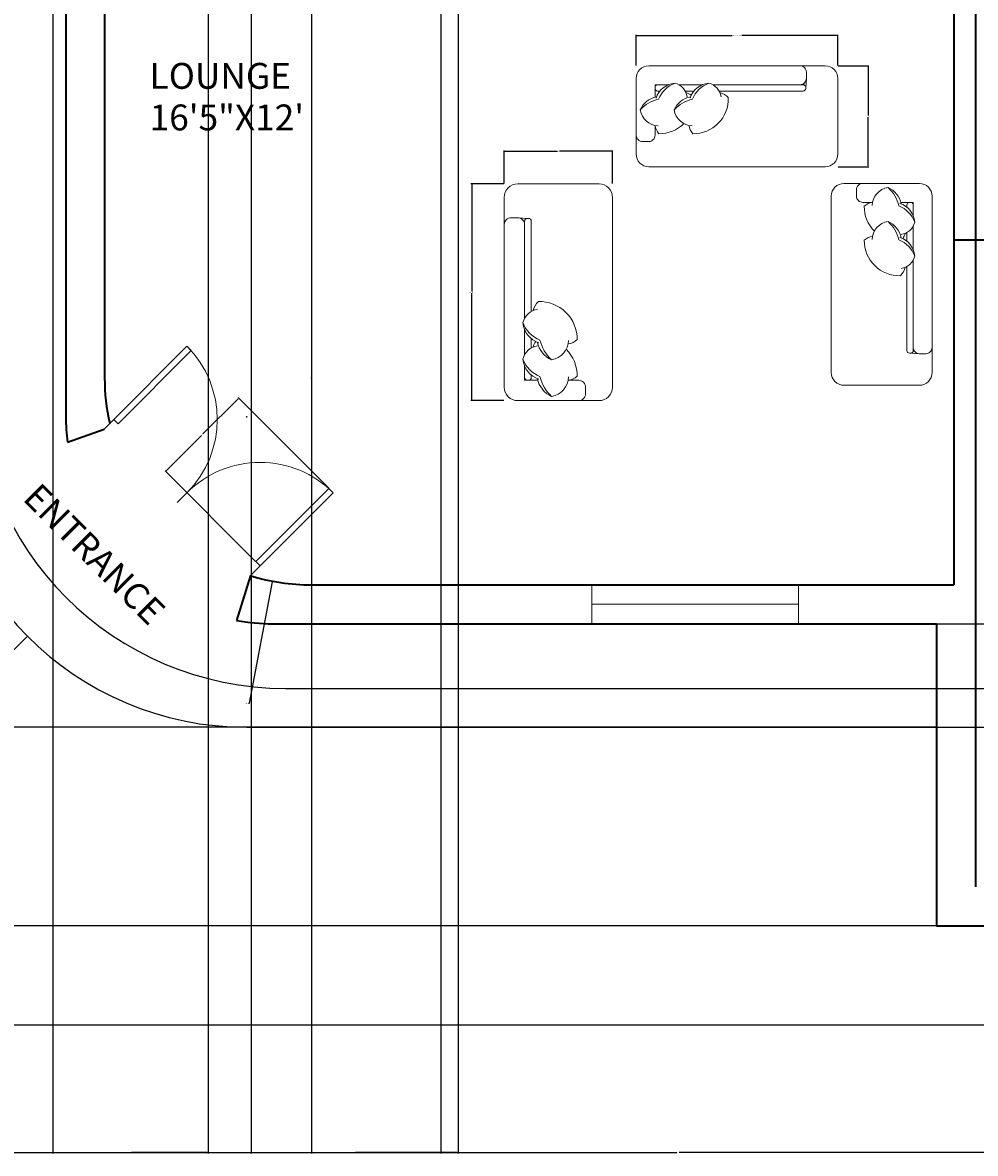
# Model space of a CAD drawing. Units: inches. Extents: x 450 to 1026, y 542 to 1190.
# Tile 4 of 11: x 586 to 807, y 542 to 804. Entities that reach past the tile are written whole.
import ezdxf

# ---------------------------------------------------------------- set-up
doc = ezdxf.new("R2010")
doc.units = ezdxf.units.IN
doc.header["$MEASUREMENT"] = 0
for name, color, linetype, lineweight in [('A-ANNO-DIMS', 2, 'Continuous', 18), ('A-AREA-IDEN', 7, 'Continuous', 18), ('A-DOOR', 4, 'Continuous', 18), ('A-FLOR', 8, 'Continuous', 25), ('A-FURN', 8, 'Continuous', 18), ('A-GLAZ', 4, 'Continuous', 18), ('A-WALL', 7, 'Continuous', 35), ('C-PROP', 7, 'Continuous', 25)]:
    doc.layers.add(name, color=color, linetype=linetype, lineweight=lineweight)
doc.styles.get("Standard").update_dxf_attribs({"font": 'arial.ttf'})
doc.dimstyles.get("Standard").update_dxf_attribs({"dimtxt": 0.18, "dimasz": 0.18, "dimexe": 0.18, "dimexo": 0.0625, "dimgap": 0.09, "dimtad": 0, "dimtih": 1, "dimtoh": 1, "dimdec": 4, "dimzin": 0, "dimdsep": 46, "dimtxsty": 'Standard', "dimcen": 0.09, "dimadec": 0, "dimazin": 0, "dimtfac": 1, "dimtdec": 4, "dimtofl": 0, "dimtmove": 0, "dimatfit": 3, "dimfxl": 1, "dimtolj": 1, "dimtzin": 0, "dimarcsym": 0})

# ---------------------------------------------------------------- blocks, each defined once
blk = doc.blocks.new('*U5')
for p, q in [((0, 0), (0, -100)), ((750, 0), (750, -100))]:
    blk.add_line(p, q)
blk.add_lwpolyline([(0, 0), (0, 750), (43.75, 750), (43.75, 0)], close=True)
blk.add_arc((0, 0), 750, 0, 90)
blk = doc.blocks.new('*U3')
for p, q in [((0, 100), (0, 0)), ((900, 100), (900, 0)), ((0, 50), (900, 50))]:
    blk.add_line(p, q)
blk = doc.blocks.new('DAY BED1')
at = {"color": 0}
blk.add_line((0.3, 0.25), (0.225, 0.2549), dxfattribs=at)
blk.add_lwpolyline([(-0.3, 0, -0.414214), (-0.4, 0.1), (-0.4, 0.1, 0.317837), (-0.4, 0.1, -0.414214), (-0.4, 0.1), (-0.4, 0.1, 1.186185), (-0.4, 0.1, -0.414214), (-0.4, 0.1), (-0.4, 1.5, -0.414214), (-0.3, 1.6), (0.3, 1.6, -0.414214), (0.4, 1.5), (0.4, 0.1, -0.414214), (0.3, 0)], format="xyb", close=True, dxfattribs=at)
for points in [[(-0.0725, 1.45), (-0.15, 1.45, -0.414214), (-0.2, 1.5), (-0.2, 1.55, -0.414214), (-0.15, 1.6)], [(-0.0756, 1.4249, -0.356772), (0.0505, 1.5682, -0.249542), (0.1543, 1.4384, 9.61688)], [(0.0505, 1.5682, -0.14773), (0.1364, 1.422, -0.213343), (0.2624, 1.2931, -0.178662)], [(-0.0725, 1.4501, 0.165541), (-0.1386, 1.4192, 0.200231), (-0.0581, 1.2207, 0.121523)], [(0.1433, 1.4422, -0.306663), (0.2624, 1.2931, -0.30633), (0.1536, 1.1957, 0.872847)], [(0.25, 1.3448), (0.25, 1.45), (0.1517, 1.45, -0.414214)], [(0.2, 1.4118), (0.2, 1.43, -0.414214), (0.22, 1.45), (0.23, 1.45, -0.414214), (0.25, 1.43)], [(0.25, 1.43), (0.25, 1.3448, -0.414214)], [(-0.0756, 1.1556, -0.356772), (0.0505, 1.2988, -0.249542), (0.1543, 1.169, 9.61688)], [(0.0505, 1.2988, -0.14773), (0.1364, 1.1527, -0.213343), (0.2624, 1.0238, -0.178662)], [(0.25, 1.2616), (0.25, 1.0755, -0.414214)], [(-0.0725, 1.1808, 0.165541), (-0.1386, 1.1498, 0.425989), (0.1479, 0.869, 0.121523), (0.1873, 0.9357, -7.115464)], [(0.1433, 1.1729, -0.306663), (0.2624, 1.0238, -0.30633), (0.1536, 0.9263, 0.872847)], [(0.1678, 1.1631, 0.071865), (0.1873, 1.205, -7.115464)], [(0.2, 1.1425), (0.2, 1.2113, -0.414214)], [(0.25, 0.9923), (0.25, 0.2749, -0.414214), (0.23, 0.2549), (0.22, 0.2549, -0.414214), (0.2, 0.2749), (0.2, 0.9419, -0.414214)], [(0.25, 0.3775), (0.25, 0.3, 0.414214), (0.3, 0.25), (0.35, 0.25, 0.414214), (0.4, 0.3)]]:
    blk.add_lwpolyline(points, format="xyb", dxfattribs=at)
for points in [[(0.25, 1.0755), (0.25, 1.2616)], [(0.25, 0.3775), (0.25, 0.9923)]]:
    blk.add_lwpolyline(points, dxfattribs=at)
blk = doc.blocks.new('*D25')
at = {"layer": 'A-ANNO-DIMS', "color": 0, "lineweight": -2, "transparency": 16777216}
for p, q in [((697.29, 766.92), (689.63, 766.92)), ((689.81, 766.74), (689.81, 741.97)), ((689.81, 716.84), (689.81, 741.61)), ((697.29, 716.66), (689.63, 716.66))]:
    blk.add_line(p, q, dxfattribs=at)
at = {"layer": 'A-ANNO-DIMS', "color": 0, "transparency": 16777216}
for points in [[(689.78, 766.74), (689.84, 766.74), (689.81, 766.92)], [(689.78, 716.84), (689.84, 716.84), (689.81, 716.66)]]:
    blk.add_solid(points, dxfattribs=at)
at = {"layer": 'Defpoints', "color": 0, "transparency": 16777216}
for p in [(697.35, 766.92), (689.81, 716.66), (697.35, 716.66)]:
    blk.add_point(p, dxfattribs=at)
at = {"layer": 'A-ANNO-DIMS', "color": 0, "transparency": 16777216, "insert": (689.81, 741.79), "char_height": 0.18, "attachment_point": 5}
blk.add_mtext('\\A1;DAY BED 50', dxfattribs=at)
blk = doc.blocks.new('*D26')
at = {"layer": 'A-ANNO-DIMS', "color": 0, "lineweight": -2, "transparency": 16777216}
for p, q in [((697.35, 766.98), (697.35, 774.64)), ((697.53, 774.46), (709.7, 774.46)), ((722.31, 774.46), (710.14, 774.46)), ((722.49, 766.98), (722.49, 774.64))]:
    blk.add_line(p, q, dxfattribs=at)
at = {"layer": 'A-ANNO-DIMS', "color": 0, "transparency": 16777216}
for points in [[(697.53, 774.49), (697.53, 774.43), (697.35, 774.46)], [(722.31, 774.49), (722.31, 774.43), (722.49, 774.46)]]:
    blk.add_solid(points, dxfattribs=at)
at = {"layer": 'Defpoints', "color": 0, "transparency": 16777216}
for p in [(697.35, 774.46), (697.35, 766.92), (722.49, 766.92)]:
    blk.add_point(p, dxfattribs=at)
at = {"layer": 'A-ANNO-DIMS', "color": 0, "transparency": 16777216, "insert": (709.92, 774.46), "char_height": 0.18, "attachment_point": 5}
blk.add_mtext('\\A1;25', dxfattribs=at)
blk = doc.blocks.new('*D27')
at = {"layer": 'A-ANNO-DIMS', "color": 0, "lineweight": -2, "transparency": 16777216}
for p, q in [((727.96, 794.34), (727.96, 801.47)), ((728.14, 801.29), (750.24, 801.29)), ((774.56, 801.29), (752.46, 801.29)), ((774.74, 794.34), (774.74, 801.47))]:
    blk.add_line(p, q, dxfattribs=at)
at = {"layer": 'A-ANNO-DIMS', "color": 0, "transparency": 16777216}
for points in [[(728.14, 801.32), (728.14, 801.26), (727.96, 801.29)], [(774.56, 801.32), (774.56, 801.26), (774.74, 801.29)]]:
    blk.add_solid(points, dxfattribs=at)
at = {"layer": 'Defpoints', "color": 0, "transparency": 16777216}
for p in [(727.96, 801.29), (727.96, 794.28), (774.74, 794.28)]:
    blk.add_point(p, dxfattribs=at)
at = {"layer": 'A-ANNO-DIMS', "color": 0, "transparency": 16777216, "insert": (751.35, 801.29), "char_height": 0.18, "attachment_point": 5}
blk.add_mtext('\\A1;DAY BED 47 TYP.', dxfattribs=at)
blk = doc.blocks.new('*D28')
at = {"layer": 'A-ANNO-DIMS', "color": 0, "lineweight": -2, "transparency": 16777216}
for p, q in [((774.81, 794.28), (781.94, 794.28)), ((781.76, 794.1), (781.76, 782.76)), ((781.76, 771.07), (781.76, 782.4)), ((774.81, 770.89), (781.94, 770.89))]:
    blk.add_line(p, q, dxfattribs=at)
at = {"layer": 'A-ANNO-DIMS', "color": 0, "transparency": 16777216}
for points in [[(781.73, 794.1), (781.79, 794.1), (781.76, 794.28)], [(781.73, 771.07), (781.79, 771.07), (781.76, 770.89)]]:
    blk.add_solid(points, dxfattribs=at)
at = {"layer": 'Defpoints', "color": 0, "transparency": 16777216}
for p in [(774.74, 794.28), (781.76, 794.28), (774.74, 770.89)]:
    blk.add_point(p, dxfattribs=at)
at = {"layer": 'A-ANNO-DIMS', "color": 0, "transparency": 16777216, "insert": (781.76, 782.58), "char_height": 0.18, "attachment_point": 5}
blk.add_mtext('\\A1;23 TYP.', dxfattribs=at)
blk = doc.blocks.new('*D45')
at = {"layer": 'A-ANNO-DIMS', "color": 0, "lineweight": -2, "transparency": 16777216}
for p, q in [((479.65, 571.88), (479.65, 542.16)), ((995.65, 571.88), (995.65, 542.16)), ((479.83, 542.34), (737.36, 542.34)), ((995.47, 542.34), (737.94, 542.34))]:
    blk.add_line(p, q, dxfattribs=at)
at = {"layer": 'A-ANNO-DIMS', "color": 0, "transparency": 16777216}
for points in [[(479.83, 542.37), (479.83, 542.31), (479.65, 542.34)], [(995.47, 542.37), (995.47, 542.31), (995.65, 542.34)]]:
    blk.add_solid(points, dxfattribs=at)
at = {"layer": 'Defpoints', "color": 0, "transparency": 16777216}
for p in [(479.65, 571.94), (995.65, 571.94), (995.65, 542.34)]:
    blk.add_point(p, dxfattribs=at)
at = {"layer": 'A-ANNO-DIMS', "color": 0, "transparency": 16777216, "insert": (737.65, 542.34), "char_height": 0.18, "attachment_point": 5}
blk.add_mtext('\\A1;516', dxfattribs=at)
blk = doc.blocks.new('*D53')
at = {"layer": 'A-ANNO-DIMS', "color": 0, "lineweight": -2, "transparency": 16777216}
for p, q in [((479.59, 817.94), (449.87, 817.94)), ((450.05, 817.76), (450.05, 706.62)), ((450.05, 595.12), (450.05, 706.26)), ((797.59, 594.94), (449.87, 594.94))]:
    blk.add_line(p, q, dxfattribs=at)
at = {"layer": 'A-ANNO-DIMS', "color": 0, "transparency": 16777216}
for points in [[(450.02, 817.76), (450.08, 817.76), (450.05, 817.94)], [(450.02, 595.12), (450.08, 595.12), (450.05, 594.94)]]:
    blk.add_solid(points, dxfattribs=at)
at = {"layer": 'Defpoints', "color": 0, "transparency": 16777216}
for p in [(479.65, 817.94), (450.05, 594.94), (797.65, 594.94)]:
    blk.add_point(p, dxfattribs=at)
at = {"layer": 'A-ANNO-DIMS', "color": 0, "transparency": 16777216, "insert": (450.05, 706.44), "char_height": 0.18, "attachment_point": 5}
blk.add_mtext('\\A1;223', dxfattribs=at)
blk = doc.blocks.new('*D54')
at = {"layer": 'A-ANNO-DIMS', "color": 0, "lineweight": -2, "transparency": 16777216}
for p, q in [((797.59, 594.94), (449.87, 594.94)), ((450.05, 594.76), (450.05, 583.62)), ((450.05, 572.12), (450.05, 583.26)), ((479.59, 571.94), (449.87, 571.94))]:
    blk.add_line(p, q, dxfattribs=at)
at = {"layer": 'A-ANNO-DIMS', "color": 0, "transparency": 16777216}
for points in [[(450.02, 594.76), (450.08, 594.76), (450.05, 594.94)], [(450.02, 572.12), (450.08, 572.12), (450.05, 571.94)]]:
    blk.add_solid(points, dxfattribs=at)
at = {"layer": 'Defpoints', "color": 0, "transparency": 16777216}
for p in [(797.65, 594.94), (450.05, 571.94), (479.65, 571.94)]:
    blk.add_point(p, dxfattribs=at)
at = {"layer": 'A-ANNO-DIMS', "color": 0, "transparency": 16777216, "insert": (450.05, 583.44), "char_height": 0.18, "attachment_point": 5}
blk.add_mtext('\\A1;23', dxfattribs=at)
blk = doc.blocks.new('*D57')
at = {"layer": 'A-ANNO-DIMS', "color": 0, "lineweight": -2, "transparency": 16777216}
for p, q in [((638.65, 970.88), (638.65, 542.16)), ((686.65, 970.88), (686.65, 542.16)), ((638.83, 542.34), (662.43, 542.34)), ((686.47, 542.34), (662.87, 542.34))]:
    blk.add_line(p, q, dxfattribs=at)
at = {"layer": 'A-ANNO-DIMS', "color": 0, "transparency": 16777216}
for points in [[(638.83, 542.37), (638.83, 542.31), (638.65, 542.34)], [(686.47, 542.37), (686.47, 542.31), (686.65, 542.34)]]:
    blk.add_solid(points, dxfattribs=at)
at = {"layer": 'Defpoints', "color": 0, "transparency": 16777216}
for p in [(638.65, 970.94), (686.65, 970.94), (686.65, 542.34)]:
    blk.add_point(p, dxfattribs=at)
at = {"layer": 'A-ANNO-DIMS', "color": 0, "transparency": 16777216, "insert": (662.65, 542.34), "char_height": 0.18, "attachment_point": 5}
blk.add_mtext('\\A1;48', dxfattribs=at)
blk = doc.blocks.new('*D64')
at = {"layer": 'A-ANNO-DIMS', "color": 0, "lineweight": -2, "transparency": 16777216}
for p, q in [((635.65, 717.11), (627.47, 708.94)), ((656.66, 696.36), (635.65, 717.37)), ((618.93, 700.4), (627.11, 708.58)), ((639.69, 679.38), (618.68, 700.4))]:
    blk.add_line(p, q, dxfattribs=at)
at = {"layer": 'A-ANNO-DIMS', "color": 0, "transparency": 16777216}
for points in [[(635.63, 717.14), (635.67, 717.09), (635.77, 717.24)], [(618.91, 700.42), (618.95, 700.38), (618.8, 700.27)]]:
    blk.add_solid(points, dxfattribs=at)
at = {"layer": 'Defpoints', "color": 0, "transparency": 16777216}
for p in [(635.77, 717.24), (656.7, 696.31), (639.73, 679.34)]:
    blk.add_point(p, dxfattribs=at)
at = {"layer": 'A-ANNO-DIMS', "color": 0, "transparency": 16777216, "insert": (627.29, 708.76), "char_height": 0.18, "attachment_point": 5}
blk.add_mtext('\\A1;24', dxfattribs=at)
blk = doc.blocks.new('*D65')
at = {"layer": 'A-ANNO-DIMS', "color": 0, "lineweight": -2, "transparency": 16777216}
for p, q in [((592.65, 970.88), (592.65, 542.16)), ((628.65, 970.88), (628.65, 542.16)), ((592.83, 542.34), (610.43, 542.34)), ((628.47, 542.34), (610.87, 542.34))]:
    blk.add_line(p, q, dxfattribs=at)
at = {"layer": 'A-ANNO-DIMS', "color": 0, "transparency": 16777216}
for points in [[(592.83, 542.37), (592.83, 542.31), (592.65, 542.34)], [(628.47, 542.37), (628.47, 542.31), (628.65, 542.34)]]:
    blk.add_solid(points, dxfattribs=at)
at = {"layer": 'Defpoints', "color": 0, "transparency": 16777216}
for p in [(592.65, 970.94), (628.65, 970.94), (628.65, 542.34)]:
    blk.add_point(p, dxfattribs=at)
at = {"layer": 'A-ANNO-DIMS', "color": 0, "transparency": 16777216, "insert": (610.65, 542.34), "char_height": 0.18, "attachment_point": 5}
blk.add_mtext('\\A1;36', dxfattribs=at)
blk = doc.blocks.new('*D66')
at = {"layer": 'A-ANNO-DIMS', "color": 0, "lineweight": -2, "transparency": 16777216}
for p, q in [((652.65, 1018.88), (652.65, 542.16)), ((682.65, 1018.88), (682.65, 542.16)), ((652.83, 542.34), (667.43, 542.34)), ((682.47, 542.34), (667.87, 542.34))]:
    blk.add_line(p, q, dxfattribs=at)
at = {"layer": 'A-ANNO-DIMS', "color": 0, "transparency": 16777216}
for points in [[(652.83, 542.37), (652.83, 542.31), (652.65, 542.34)], [(682.47, 542.37), (682.47, 542.31), (682.65, 542.34)]]:
    blk.add_solid(points, dxfattribs=at)
at = {"layer": 'Defpoints', "color": 0, "transparency": 16777216}
for p in [(652.65, 1018.94), (682.65, 1018.94), (682.65, 542.34)]:
    blk.add_point(p, dxfattribs=at)
at = {"layer": 'A-ANNO-DIMS', "color": 0, "transparency": 16777216, "insert": (667.65, 542.34), "char_height": 0.18, "attachment_point": 5}
blk.add_mtext('\\A1;30', dxfattribs=at)
blk = doc.blocks.new('*D70')
at = {"layer": 'A-ANNO-DIMS', "color": 0, "lineweight": -2, "transparency": 16777216}
for p, q in [((565.65, 713.01), (565.65, 1189.72)), ((565.83, 1189.54), (580.43, 1189.54)), ((595.47, 1189.54), (580.87, 1189.54)), ((595.65, 713.01), (595.65, 1189.72))]:
    blk.add_line(p, q, dxfattribs=at)
at = {"layer": 'A-ANNO-DIMS', "color": 0, "transparency": 16777216}
for points in [[(565.83, 1189.57), (565.83, 1189.51), (565.65, 1189.54)], [(595.47, 1189.57), (595.47, 1189.51), (595.65, 1189.54)]]:
    blk.add_solid(points, dxfattribs=at)
at = {"layer": 'Defpoints', "color": 0, "transparency": 16777216}
for p in [(595.65, 1189.54), (565.65, 712.94), (595.65, 712.94)]:
    blk.add_point(p, dxfattribs=at)
at = {"layer": 'A-ANNO-DIMS', "color": 0, "transparency": 16777216, "insert": (580.65, 1189.54), "char_height": 0.18, "attachment_point": 5}
blk.add_mtext('\\A1;30', dxfattribs=at)
blk = doc.blocks.new('*D71')
at = {"layer": 'A-ANNO-DIMS', "color": 0, "lineweight": -2, "transparency": 16777216}
for p, q in [((646.71, 649.94), (1025.43, 649.94)), ((1025.25, 649.76), (1025.25, 645.62)), ((1025.25, 641.12), (1025.25, 645.26)), ((637.71, 640.94), (1025.43, 640.94))]:
    blk.add_line(p, q, dxfattribs=at)
at = {"layer": 'A-ANNO-DIMS', "color": 0, "transparency": 16777216}
for points in [[(1025.22, 649.76), (1025.28, 649.76), (1025.25, 649.94)], [(1025.22, 641.12), (1025.28, 641.12), (1025.25, 640.94)]]:
    blk.add_solid(points, dxfattribs=at)
at = {"layer": 'Defpoints', "color": 0, "transparency": 16777216}
for p in [(646.65, 649.94), (1025.25, 649.94), (637.65, 640.94)]:
    blk.add_point(p, dxfattribs=at)
at = {"layer": 'A-ANNO-DIMS', "color": 0, "transparency": 16777216, "insert": (1025.25, 645.44), "char_height": 0.18, "attachment_point": 5}
blk.add_mtext('\\A1;9', dxfattribs=at)
blk = doc.blocks.new('*D72')
at = {"layer": 'A-ANNO-DIMS', "color": 0, "lineweight": -2, "transparency": 16777216}
for p, q in [((643.71, 664.94), (1025.43, 664.94)), ((1025.25, 664.76), (1025.25, 653.12)), ((1025.25, 641.12), (1025.25, 652.76)), ((637.71, 640.94), (1025.43, 640.94))]:
    blk.add_line(p, q, dxfattribs=at)
at = {"layer": 'A-ANNO-DIMS', "color": 0, "transparency": 16777216}
for points in [[(1025.22, 664.76), (1025.28, 664.76), (1025.25, 664.94)], [(1025.22, 641.12), (1025.28, 641.12), (1025.25, 640.94)]]:
    blk.add_solid(points, dxfattribs=at)
at = {"layer": 'Defpoints', "color": 0, "transparency": 16777216}
for p in [(643.65, 664.94), (1025.25, 664.94), (637.65, 640.94)]:
    blk.add_point(p, dxfattribs=at)
at = {"layer": 'A-ANNO-DIMS', "color": 0, "transparency": 16777216, "insert": (1025.25, 652.94), "char_height": 0.18, "attachment_point": 5}
blk.add_mtext('\\A1;24', dxfattribs=at)
blk = doc.blocks.new('*D73')
at = {"layer": 'A-ANNO-DIMS', "color": 0, "lineweight": -2, "transparency": 16777216}
for p, q in [((797.59, 640.94), (449.87, 640.94)), ((450.05, 640.76), (450.05, 618.12)), ((450.05, 595.12), (450.05, 617.76)), ((797.59, 594.94), (449.87, 594.94))]:
    blk.add_line(p, q, dxfattribs=at)
at = {"layer": 'A-ANNO-DIMS', "color": 0, "transparency": 16777216}
for points in [[(450.02, 640.76), (450.08, 640.76), (450.05, 640.94)], [(450.02, 595.12), (450.08, 595.12), (450.05, 594.94)]]:
    blk.add_solid(points, dxfattribs=at)
at = {"layer": 'Defpoints', "color": 0, "transparency": 16777216}
for p in [(450.05, 640.94), (797.65, 640.94), (797.65, 594.94)]:
    blk.add_point(p, dxfattribs=at)
at = {"layer": 'A-ANNO-DIMS', "color": 0, "transparency": 16777216, "insert": (450.05, 617.94), "char_height": 0.18, "attachment_point": 5}
blk.add_mtext('\\A1;46', dxfattribs=at)
blk = doc.blocks.new('*D75')
at = {"layer": 'A-ANNO-DIMS', "color": 0, "lineweight": -2, "transparency": 16777216}
for p, q in [((637.65, 712.85), (637.65, 713.03)), ((637.56, 712.94), (637.74, 712.94)), ((556.19, 631.48), (586.61, 661.9)), ((556.01, 631.48), (556.19, 631.48))]:
    blk.add_line(p, q, dxfattribs=at)
at = {"layer": 'A-ANNO-DIMS', "color": 0, "transparency": 16777216}
blk.add_solid([(586.59, 661.92), (586.63, 661.88), (586.74, 662.03)], dxfattribs=at)
at = {"layer": 'Defpoints', "color": 0, "transparency": 16777216}
for p in [(637.65, 712.94), (586.74, 662.03)]:
    blk.add_point(p, dxfattribs=at)
at = {"layer": 'A-ANNO-DIMS', "color": 0, "transparency": 16777216, "insert": (555.51, 631.48), "char_height": 0.18, "attachment_point": 5}
blk.add_mtext('\\A1;2X R72', dxfattribs=at)
blk = doc.blocks.new('*D76')
at = {"layer": 'A-ANNO-DIMS', "color": 0, "lineweight": -2, "transparency": 16777216}
for p, q in [((652.56, 721.94), (652.74, 721.94)), ((652.65, 721.85), (652.65, 722.03)), ((638.25, 646.5), (643.62, 674.62)), ((638.07, 646.5), (638.25, 646.5))]:
    blk.add_line(p, q, dxfattribs=at)
at = {"layer": 'A-ANNO-DIMS', "color": 0, "transparency": 16777216}
blk.add_solid([(643.59, 674.62), (643.65, 674.61), (643.65, 674.79)], dxfattribs=at)
at = {"layer": 'Defpoints', "color": 0, "transparency": 16777216}
for p in [(652.65, 721.94), (643.65, 674.79)]:
    blk.add_point(p, dxfattribs=at)
at = {"layer": 'A-ANNO-DIMS', "color": 0, "transparency": 16777216, "insert": (637.57, 646.5), "char_height": 0.18, "attachment_point": 5}
blk.add_mtext('\\A1;4X R48', dxfattribs=at)

msp = doc.modelspace()

# ---------------------------------------------------------------- linework, layer by layer
at = {"layer": 'A-FLOR'}
for points in [[(565.6513, 826.9426), (565.6513, 712.9426, 0.41421356), (637.6513, 640.9426), (797.6513, 640.9426)], [(574.6513, 826.9426), (574.6513, 721.9426, 0.41421356), (646.6513, 649.9426), (797.6513, 649.9426)]]:
    msp.add_lwpolyline(points, format="xyb", dxfattribs=at)
at = {"layer": 'A-GLAZ'}
msp.add_line((765.6513, 673.9426), (765.6513, 664.9426), dxfattribs=at)
msp.add_lwpolyline([(765.6513, 664.9426), (717.6513, 664.9426), (717.6513, 673.9426)], dxfattribs=at)
at = {"layer": 'A-WALL'}
for p, q in [((801.6513, 826.9426), (801.6513, 673.9426)), ((806.6513, 826.9426), (806.6513, 603.9426)), ((801.6513, 753.9426), (810.6513, 753.9426)), ((596.021, 706.9969), (604.5204, 710.029)), ((638.4615, 676.0879), (635.2811, 665.678)), ((797.6513, 664.9426), (797.6513, 594.9426)), ((797.6513, 594.9426), (959.6513, 594.9426))]:
    msp.add_line(p, q, dxfattribs=at)
for points in [[(595.6513, 826.9426), (595.6513, 712.9426, 0.03105652), (596.021, 706.9969, 0.03105652)], [(604.6513, 826.9426), (604.6513, 721.9426, 0.0557141), (605.8359, 711.3446, 0.0557141)], [(638.4615, 676.0879, 0.07516745), (652.6513, 673.9426), (801.6513, 673.9426)], [(635.2811, 665.678, 0.04384727), (643.6513, 664.9426), (797.6513, 664.9426)]]:
    msp.add_lwpolyline(points, format="xyb", dxfattribs=at)
at = {"layer": 'C-PROP'}
msp.add_line((479.6513, 571.9426), (995.6513, 571.9426), dxfattribs=at)

# ---------------------------------------------------------------- block references
at = {"layer": 'A-DOOR', "yscale": 0.032, "zscale": 0.032, "rotation": 315}
for p, xscale in [((606.7832, 712.2918), 0.032), ((640.7243, 678.3506), -0.032)]:
    msp.add_blockref('*U5', p, dxfattribs=dict(at, xscale=xscale))
at = {"layer": 'A-FURN', "ltscale": 0.03}
for p, xscale, yscale, zscale, rotation in [((774.7435, 782.5808), 29.23701563285006, 29.23701563285006, 29.23701563285006, 89.99999999999999), ((709.9204, 766.9208), 31.41507934722368, 31.41507934722368, 31.41507934722368, 180)]:
    msp.add_blockref('DAY BED1', p, dxfattribs=dict(at, xscale=xscale, yscale=yscale, zscale=zscale, rotation=rotation))
at = {"layer": 'A-FURN', "ltscale": 0.03, "xscale": 29.23701563285006, "yscale": 29.23701563285006, "zscale": 29.23701563285006}
msp.add_blockref('DAY BED1', (784.9159, 720.2202), dxfattribs=at)
at = {"layer": 'A-GLAZ', "xscale": 0.0533333333333333, "yscale": 0.0533333333333333, "zscale": 0.0533333333333333}
msp.add_blockref('*U3', (717.6513, 666.7759), dxfattribs=at)

# ---------------------------------------------------------------- texts
at = {"layer": 'A-AREA-IDEN'}
for s, p in [('LOUNGE', (615.089, 788.944)), ('16\'5"X12\'', (615.089, 779.3055))]:
    msp.add_text(s, height=6, dxfattribs=at).set_placement(p)
msp.add_text('ENTRANCE', height=6, rotation=315, dxfattribs=at).set_placement((585.409, 693.7615))

# ---------------------------------------------------------------- dimensions: what is measured, and where the dimension line sits
at = {"layer": 'A-ANNO-DIMS'}
for base, p1, p2, picture, middle in [((595.6513, 1189.5426), (565.6513, 712.9426), (595.6513, 712.9426), '*D70', (580.6513, 1189.5426)), ((682.6513, 542.3426), (652.6513, 1018.9426), (682.6513, 1018.9426), '*D66', (667.6513, 542.3426)), ((628.6513, 542.3426), (592.6513, 970.9426), (628.6513, 970.9426), '*D65', (610.6513, 542.3426)), ((686.6513, 542.3426), (638.6513, 970.9426), (686.6513, 970.9426), '*D57', (662.6513, 542.3426)), ((995.6513, 542.3426), (479.6513, 571.9426), (995.6513, 571.9426), '*D45', (737.6513, 542.3426))]:
    dim = msp.add_linear_dim(base=base, p1=p1, p2=p2, dimstyle='Standard', override={"dimdec": 0, "dimlfac": 1, "dimrnd": 0, "dimzin": 0, "dimdsep": 46, "dimlunit": 2}, dxfattribs=at)
    dim.commit()
    dim.dimension.update_dxf_attribs({"geometry": picture, "text_midpoint": middle})
for base, p1, p2, angle, picture, middle in [((450.0513, 594.9426), (479.6513, 817.9426), (797.6513, 594.9426), 90, '*D53', (450.0513, 706.4426)), ((697.3544, 774.4604), (722.4864, 766.9208), (697.3544, 766.9208), 180, '*D26', (709.9204, 774.4604)), ((635.7745, 717.2415), (639.7343, 679.3406), (656.7049, 696.3112), 45, '*D64', (627.2893, 708.7562)), ((1025.2513, 664.9426), (637.6513, 640.9426), (643.6513, 664.9426), 90, '*D72', (1025.2513, 652.9426)), ((1025.2513, 649.9426), (637.6513, 640.9426), (646.6513, 649.9426), 90, '*D71', (1025.2513, 645.4426)), ((450.0513, 640.9426), (797.6513, 594.9426), (797.6513, 640.9426), 90, '*D73', (450.0513, 617.9426)), ((450.0513, 571.9426), (797.6513, 594.9426), (479.6513, 571.9426), 90, '*D54', (450.0513, 583.4426))]:
    dim = msp.add_linear_dim(base=base, p1=p1, p2=p2, angle=angle, dimstyle='Standard', override={"dimdec": 0, "dimlfac": 1, "dimrnd": 0, "dimzin": 0, "dimdsep": 46, "dimlunit": 2}, dxfattribs=at)
    dim.commit()
    dim.dimension.update_dxf_attribs({"geometry": picture, "text_midpoint": middle})
for base, p1, p2, angle, text, picture, middle in [((727.9642, 801.2925), (774.7435, 794.2757), (727.9642, 794.2757), 180, 'DAY BED <> TYP.', '*D27', (751.3538, 801.2925)), ((781.7603, 794.2757), (774.7435, 770.886), (774.7435, 794.2757), 90, '<> TYP.', '*D28', (781.7603, 782.5808)), ((689.8148, 716.6567), (697.3544, 766.9208), (697.3544, 716.6567), 270, 'DAY BED <>', '*D25', (689.8148, 741.7887))]:
    dim = msp.add_linear_dim(base=base, p1=p1, p2=p2, angle=angle, text=text, dimstyle='Standard', override={"dimdec": 0, "dimlfac": 1, "dimrnd": 0, "dimzin": 0, "dimdsep": 46, "dimlunit": 2}, dxfattribs=at)
    dim.commit()
    dim.dimension.update_dxf_attribs({"geometry": picture, "text_midpoint": middle})
for center, mpoint, text, picture, middle in [((652.6513, 721.9426), (643.6508, 674.794), '4X <>', '*D76', (637.5682, 646.5048)), ((637.6513, 712.9426), (586.7403, 662.0303), '2X <>', '*D75', (555.5146, 631.4829))]:
    dim = msp.add_radius_dim(center=center, mpoint=mpoint, text=text, dimstyle='Standard', override={"dimdec": 0, "dimlfac": 1, "dimrnd": 0, "dimzin": 0, "dimdsep": 46, "dimlunit": 2}, dxfattribs=at)
    dim.commit()
    dim.dimension.update_dxf_attribs({"geometry": picture, "text_midpoint": middle, "dimtype": 164})

doc.saveas('drawing.dxf')
